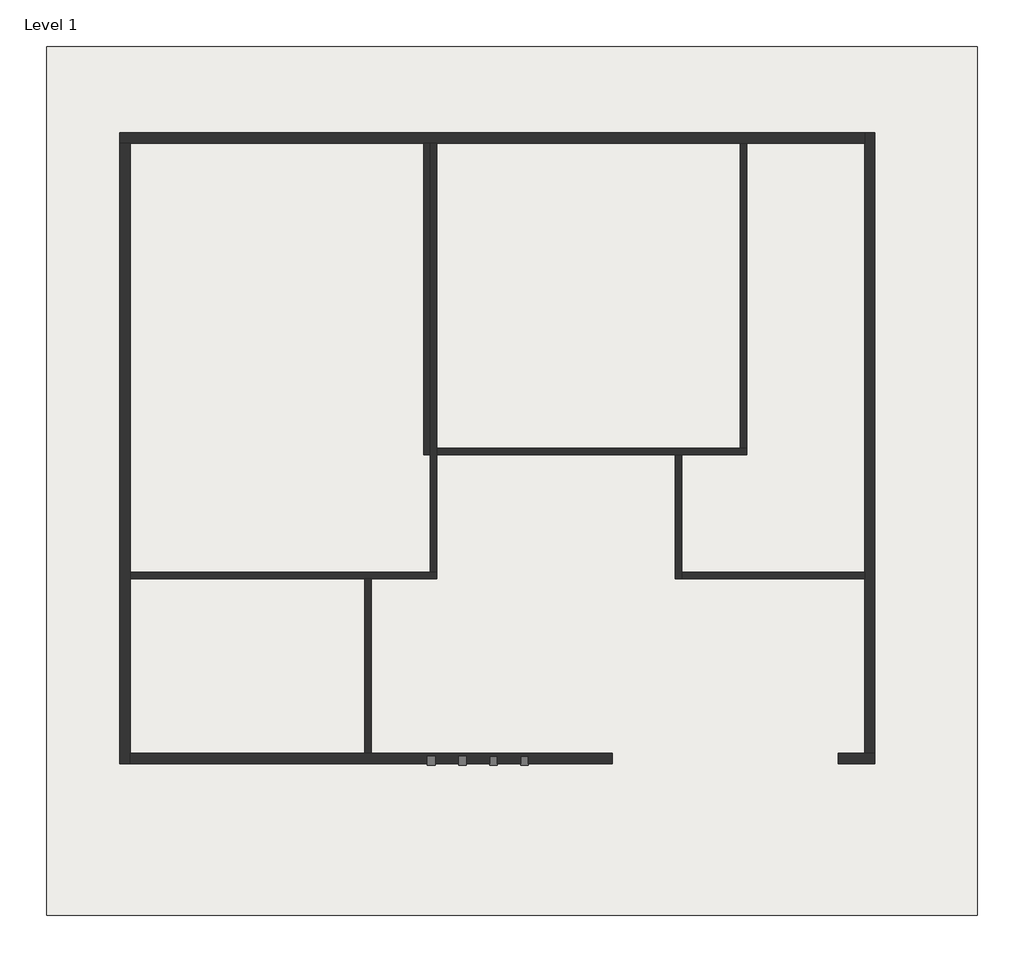
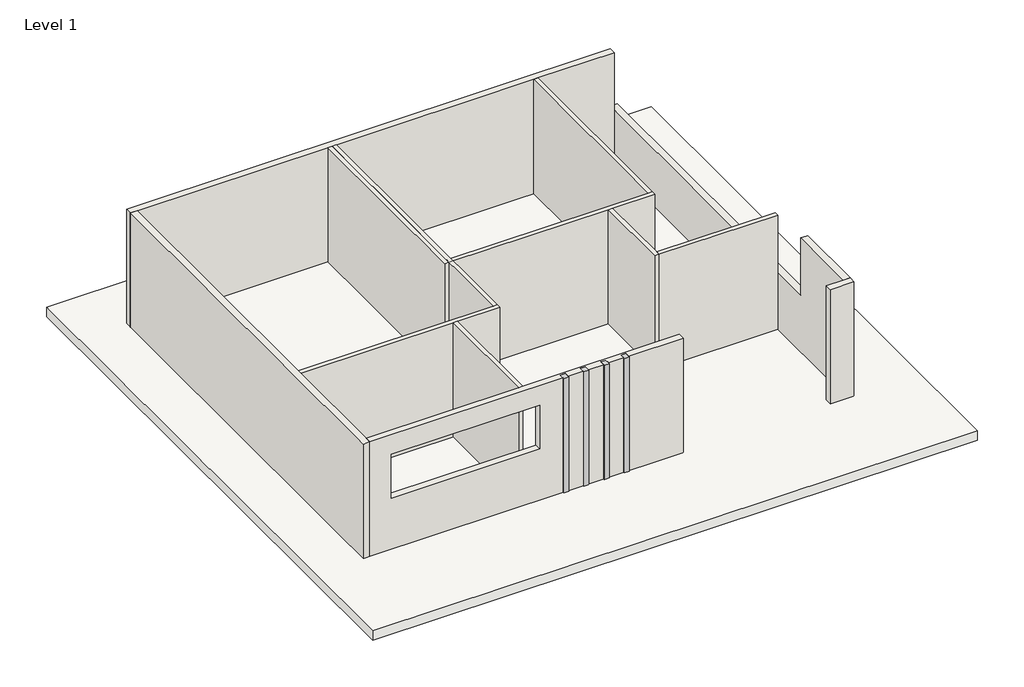
# One storey: 12 walls, 4 proxies, 1 slab.
"""IFC4 building model written with IfcOpenShell, lengths in millimetres."""

from ifc_helpers import new_model, si_unit, frame, origin, origin_with_axes, place, context, project, spatial, polyline, outline, extrude, faceted_brep, element, save

model = new_model("IFC4")

# Units and contexts
model_context = context("Model", 3, world=origin())
ifc_project = project(units=[si_unit("LENGTHUNIT", "METRE", prefix="MILLI")], contexts=[model_context])

# Site, building, storey
site = spatial("IfcSite", under=ifc_project)
building = spatial("IfcBuilding", under=site)
storey = spatial("IfcBuildingStorey", under=building, Name="Level 1", Elevation=0.0)

# Proxies
placement = place(None, origin())
element("IfcBuildingElementProxy", 1, Name="Reveal", ObjectType="Reveal", at=placement, inside=storey, context=model_context, shape_type="SweptSolid", body=[
    extrude(outline(polyline([(-2724.5749149, -2415.4251257), (-2724.5749149, -2232.5451257), (-2572.1749149, -2232.5451257), (-2572.1749149, -2415.4251257), (-2724.5749149, -2415.4251257)])), origin_with_axes(), (0.0, 0.0, 1.0), 3657.6),
])
element("IfcBuildingElementProxy", 2, Name="Reveal", ObjectType="Reveal", at=placement, inside=storey, context=model_context, shape_type="SweptSolid", body=[
    extrude(outline(polyline([(-2114.9749149, -2415.4251257), (-2114.9749149, -2232.5451257), (-1962.5749149, -2232.5451257), (-1962.5749149, -2415.4251257), (-2114.9749149, -2415.4251257)])), origin_with_axes(), (0.0, 0.0, 1.0), 3657.6),
])
element("IfcBuildingElementProxy", 3, Name="Reveal", ObjectType="Reveal", at=placement, inside=storey, context=model_context, shape_type="SweptSolid", body=[
    extrude(outline(polyline([(-1505.3749149, -2415.4251257), (-1505.3749149, -2232.5451257), (-1352.9749149, -2232.5451257), (-1352.9749149, -2415.4251257), (-1505.3749149, -2415.4251257)])), origin_with_axes(), (0.0, 0.0, 1.0), 3657.6),
])
element("IfcBuildingElementProxy", 4, Name="Reveal", ObjectType="Reveal", at=placement, inside=storey, context=model_context, shape_type="SweptSolid", body=[
    extrude(outline(polyline([(-895.7749149, -2415.4251257), (-895.7749149, -2232.5451257), (-743.3749149, -2232.5451257), (-743.3749149, -2415.4251257), (-895.7749149, -2415.4251257)])), origin_with_axes(), (0.0, 0.0, 1.0), 3657.6),
])

# Slab
element("IfcSlab", 5, ObjectType="Generic - 12\"", at=placement, inside=storey, context=model_context, shape_type="SweptSolid", body=[
    extrude(outline(polyline([(8079.4752863, 11705.7296395), (8079.4752863, -5363.0703605), (-10208.5247137, -5363.0703605), (-10208.5247137, 11705.7296395), (8079.4752863, 11705.7296395)])), frame((0.0, 0.0, -304.8), z_axis=(0.0, 0.0, 1.0), x_axis=(1.0, 0.0, 0.0)), (0.0, 0.0, 1.0), 304.8),
])

# Walls
element("IfcWall", 6, ObjectType="Generic - 5\"", at=placement, inside=storey, context=model_context, shape_type="Brep", body=[
    faceted_brep([(-8566.5749149, 1247.2548743, 0.0), (-3956.4749149, 1247.2548743, 0.0), (-3829.4749149, 1247.2548743, 0.0), (-2546.7749149, 1247.2548743, 0.0), (-2546.7749149, 1247.2548743, 3657.6), (-3829.4749149, 1247.2548743, 3657.6), (-3956.4749149, 1247.2548743, 3657.6), (-8566.5749149, 1247.2548743, 3657.6), (-8566.5749149, 1374.2548743, 0.0), (-8566.5749149, 1374.2548743, 3657.6), (-2673.7749149, 1374.2548743, 3657.6), (-2546.7749149, 1374.2548743, 3657.6), (-2546.7749149, 1374.2548743, 0.0), (-2673.7749149, 1374.2548743, 0.0)], [[[0, 1, 2, 3, 4, 5, 6, 7]], [[8, 9, 10, 11, 12, 13]], [[3, 2, 1, 0, 8, 13, 12]], [[7, 6, 5, 4, 11, 10, 9]], [[0, 7, 9, 8]], [[4, 3, 12, 11]]]),
])
element("IfcWall", 7, ObjectType="Generic - 5\"", at=placement, inside=storey, context=model_context, shape_type="SweptSolid", body=[
    extrude(outline(polyline([(-2546.7749149, 9807.0548743), (-2546.7749149, 1374.2548743), (-2673.7749149, 1374.2548743), (-2673.7749149, 9807.0548743), (-2546.7749149, 9807.0548743)])), origin_with_axes(), (0.0, 0.0, 1.0), 3657.6),
])
element("IfcWall", 8, ObjectType="Generic - 5\"", at=placement, inside=storey, context=model_context, shape_type="Brep", body=[
    faceted_brep([(-2800.7749149, 9807.0548743, 0.0), (-2800.7749149, 3685.6548743, 0.0), (-2800.7749149, 3685.6548743, 3657.6), (-2800.7749149, 9807.0548743, 3657.6), (-2673.7749149, 9807.0548743, 0.0), (-2673.7749149, 9807.0548743, 3657.6), (-2673.7749149, 3812.6548743, 3657.6), (-2673.7749149, 3685.6548743, 3657.6), (-2673.7749149, 3685.6548743, 0.0), (-2673.7749149, 3812.6548743, 0.0)], [[[0, 1, 2, 3]], [[4, 5, 6, 7, 8, 9]], [[1, 0, 4, 9, 8]], [[3, 2, 7, 6, 5]], [[0, 3, 5, 4]], [[2, 1, 8, 7]]]),
])
element("IfcWall", 9, ObjectType="Generic - 5\"", at=placement, inside=storey, context=model_context, shape_type="Brep", body=[
    faceted_brep([(-2673.7749149, 3685.6548743, 0.0), (2139.5250851, 3685.6548743, 0.0), (2266.5250851, 3685.6548743, 0.0), (3549.2250851, 3685.6548743, 0.0), (3549.2250851, 3685.6548743, 3657.6), (2266.5250851, 3685.6548743, 3657.6), (2139.5250851, 3685.6548743, 3657.6), (-2673.7749149, 3685.6548743, 3657.6), (-2673.7749149, 3812.6548743, 0.0), (-2673.7749149, 3812.6548743, 3657.6), (3422.2250851, 3812.6548743, 3657.6), (3549.2250851, 3812.6548743, 3657.6), (3549.2250851, 3812.6548743, 0.0), (3422.2250851, 3812.6548743, 0.0)], [[[0, 1, 2, 3, 4, 5, 6, 7]], [[8, 9, 10, 11, 12, 13]], [[3, 2, 1, 0, 8, 13, 12]], [[7, 6, 5, 4, 11, 10, 9]], [[0, 7, 9, 8]], [[4, 3, 12, 11]]]),
])
element("IfcWall", 10, ObjectType="Generic - 5\"", at=placement, inside=storey, context=model_context, shape_type="SweptSolid", body=[
    extrude(outline(polyline([(3549.2250851, 9807.0548743), (3549.2250851, 3812.6548743), (3422.2250851, 3812.6548743), (3422.2250851, 9807.0548743), (3549.2250851, 9807.0548743)])), origin_with_axes(), (0.0, 0.0, 1.0), 3657.6),
])
element("IfcWall", 11, ObjectType="Generic - 5\"", at=placement, inside=storey, context=model_context, shape_type="Brep", body=[
    faceted_brep([(2139.5250851, 3685.6548743, 0.0), (2139.5250851, 1247.2548743, 0.0), (2139.5250851, 1247.2548743, 3657.6), (2139.5250851, 3685.6548743, 3657.6), (2266.5250851, 3685.6548743, 0.0), (2266.5250851, 3685.6548743, 3657.6), (2266.5250851, 1374.2548743, 3657.6), (2266.5250851, 1247.2548743, 3657.6), (2266.5250851, 1247.2548743, 0.0), (2266.5250851, 1374.2548743, 0.0)], [[[0, 1, 2, 3]], [[4, 5, 6, 7, 8, 9]], [[1, 0, 4, 9, 8]], [[3, 2, 7, 6, 5]], [[0, 3, 5, 4]], [[2, 1, 8, 7]]]),
])
element("IfcWall", 12, ObjectType="Generic - 5\"", at=placement, inside=storey, context=model_context, shape_type="SweptSolid", body=[
    extrude(outline(polyline([(5860.6250851, 1247.2548743), (2266.5250851, 1247.2548743), (2266.5250851, 1374.2548743), (5860.6250851, 1374.2548743), (5860.6250851, 1247.2548743)])), origin_with_axes(), (0.0, 0.0, 1.0), 3657.6),
])
element("IfcWall", 13, ObjectType="Generic - 5\"", at=placement, inside=storey, context=model_context, shape_type="SweptSolid", body=[
    extrude(outline(polyline([(-3829.4749149, 1247.2548743), (-3829.4749149, -2181.7451257), (-3956.4749149, -2181.7451257), (-3956.4749149, 1247.2548743), (-3829.4749149, 1247.2548743)])), origin_with_axes(), (0.0, 0.0, 1.0), 3657.6),
])
element("IfcWall", 14, ObjectType="Generic - 8\"", at=placement, inside=storey, context=model_context, shape_type="Brep", body=[
    faceted_brep([(-8769.7749149, 9807.0548743, 0.0), (-8566.5749149, 9807.0548743, 0.0), (-2800.7749149, 9807.0548743, 0.0), (-2673.7749149, 9807.0548743, 0.0), (3422.2250851, 9807.0548743, 0.0), (3549.2250851, 9807.0548743, 0.0), (5860.6250851, 9807.0548743, 0.0), (5860.6250851, 9807.0548743, 3657.6), (3549.2250851, 9807.0548743, 3657.6), (3422.2250851, 9807.0548743, 3657.6), (-2673.7749149, 9807.0548743, 3657.6), (-2800.7749149, 9807.0548743, 3657.6), (-8566.5749149, 9807.0548743, 3657.6), (-8769.7749149, 9807.0548743, 3657.6), (-8769.7749149, 10010.2548743, 0.0), (-8769.7749149, 10010.2548743, 3657.6), (5860.6250851, 10010.2548743, 3657.6), (5860.6250851, 10010.2548743, 1828.8), (5860.6250851, 10010.2548743, 0.0)], [[[0, 1, 2, 3, 4, 5, 6, 7, 8, 9, 10, 11, 12, 13]], [[14, 15, 16, 17, 18]], [[6, 5, 4, 3, 2, 1, 0, 14, 18]], [[0, 13, 15, 14]], [[7, 6, 18, 17, 16]], [[13, 12, 11, 10, 9, 8, 7, 16, 15]]]),
])
element("IfcWall", 15, ObjectType="Generic - 8\"", at=placement, inside=storey, context=model_context, shape_type="Brep", body=[
    faceted_brep([(-8566.5749149, -2384.9451257, 0.0), (-8566.5749149, -2181.7451257, 0.0), (-8566.5749149, 1247.2548743, 0.0), (-8566.5749149, 1374.2548743, 0.0), (-8566.5749149, 9807.0548743, 0.0), (-8566.5749149, 9807.0548743, 3657.6), (-8566.5749149, 1374.2548743, 3657.6), (-8566.5749149, 1247.2548743, 3657.6), (-8566.5749149, -2181.7451257, 3657.6), (-8566.5749149, -2384.9451257, 3657.6), (-8769.7749149, -2384.9451257, 0.0), (-8769.7749149, -2384.9451257, 3657.6), (-8769.7749149, 9807.0548743, 3657.6), (-8769.7749149, 9807.0548743, 0.0)], [[[0, 1, 2, 3, 4, 5, 6, 7, 8, 9]], [[10, 11, 12, 13]], [[4, 3, 2, 1, 0, 10, 13]], [[0, 9, 11, 10]], [[5, 4, 13, 12]], [[9, 8, 7, 6, 5, 12, 11]]]),
])
element("IfcWall", 16, ObjectType="Generic - 8\"", at=placement, inside=storey, context=model_context, shape_type="Brep", body=[
    faceted_brep([(-8566.5749149, -2181.7451257, 0.0), (-8566.5749149, -2181.7451257, 3657.6), (-3956.4749149, -2181.7451257, 3657.6), (-3829.4749149, -2181.7451257, 3657.6), (907.6250851, -2181.7451257, 3657.6), (907.6250851, -2181.7451257, 0.0), (-3829.4749149, -2181.7451257, 0.0), (-3956.4749149, -2181.7451257, 0.0), (-3435.7749149, -2181.7451257, 3037.1162749), (-7920.2332055, -2181.7451257, 3037.1162749), (-7920.2332055, -2181.7451257, 1637.4264186), (-3435.7749149, -2181.7451257, 1637.4264186), (-8566.5749149, -2384.9451257, 3657.6), (-8566.5749149, -2384.9451257, 0.0), (-2724.5749149, -2384.9451257, 0.0), (-2724.5749149, -2384.9451257, 3657.6), (-7920.2332055, -2384.9451257, 3037.1162749), (-3435.7749149, -2384.9451257, 3037.1162749), (-3435.7749149, -2384.9451257, 1637.4264186), (-7920.2332055, -2384.9451257, 1637.4264186), (-2572.1749149, -2384.9451257, 3657.6), (-2572.1749149, -2384.9451257, 0.0), (-2114.9749149, -2384.9451257, 0.0), (-2114.9749149, -2384.9451257, 3657.6), (-1962.5749149, -2384.9451257, 3657.6), (-1962.5749149, -2384.9451257, 0.0), (-1505.3749149, -2384.9451257, 0.0), (-1505.3749149, -2384.9451257, 3657.6), (-1352.9749149, -2384.9451257, 3657.6), (-1352.9749149, -2384.9451257, 0.0), (-895.7749149, -2384.9451257, 0.0), (-895.7749149, -2384.9451257, 3657.6), (907.6250851, -2384.9451257, 0.0), (907.6250851, -2384.9451257, 3657.6), (-743.3749149, -2384.9451257, 3657.6), (-743.3749149, -2384.9451257, 0.0), (-2724.5749149, -2232.5451257, 0.0), (-2724.5749149, -2232.5451257, 3657.6), (-2572.1749149, -2232.5451257, 0.0), (-2572.1749149, -2232.5451257, 3657.6), (-2114.9749149, -2232.5451257, 0.0), (-2114.9749149, -2232.5451257, 3657.6), (-1962.5749149, -2232.5451257, 0.0), (-1962.5749149, -2232.5451257, 3657.6), (-1505.3749149, -2232.5451257, 0.0), (-1505.3749149, -2232.5451257, 3657.6), (-1352.9749149, -2232.5451257, 0.0), (-1352.9749149, -2232.5451257, 3657.6), (-895.7749149, -2232.5451257, 0.0), (-895.7749149, -2232.5451257, 3657.6), (-743.3749149, -2232.5451257, 0.0), (-743.3749149, -2232.5451257, 3657.6)], [[[0, 1, 2, 3, 4, 5, 6, 7], [8, 9, 10, 11]], [[12, 13, 14, 15], [16, 17, 18, 19]], [[20, 21, 22, 23]], [[24, 25, 26, 27]], [[28, 29, 30, 31]], [[32, 33, 34, 35]], [[1, 0, 13, 12]], [[9, 8, 17, 16]], [[10, 9, 16, 19]], [[11, 10, 19, 18]], [[8, 11, 18, 17]], [[36, 37, 15, 14]], [[37, 36, 38, 39]], [[39, 38, 21, 20]], [[40, 41, 23, 22]], [[41, 40, 42, 43]], [[43, 42, 25, 24]], [[44, 45, 27, 26]], [[45, 44, 46, 47]], [[47, 46, 29, 28]], [[48, 49, 31, 30]], [[49, 48, 50, 51]], [[51, 50, 35, 34]], [[5, 4, 33, 32]], [[0, 7, 6, 5, 32, 35, 50, 48, 30, 29, 46, 44, 26, 25, 42, 40, 22, 21, 38, 36, 14, 13]], [[4, 3, 2, 1, 12, 15, 37, 39, 20, 23, 41, 43, 24, 27, 45, 47, 28, 31, 49, 51, 34, 33]]]),
    faceted_brep([(6063.8250851, -2181.7451257, 3657.6), (6063.8250851, -2181.7451257, 0.0), (5860.6250851, -2181.7451257, 0.0), (5347.1745768, -2181.7451257, 0.0), (5347.1745768, -2181.7451257, 3657.6), (5860.6250851, -2181.7451257, 3657.6), (6063.8250851, -2384.9451257, 0.0), (6063.8250851, -2384.9451257, 3657.6), (5347.1745768, -2384.9451257, 3657.6), (5347.1745768, -2384.9451257, 0.0)], [[[0, 1, 2, 3, 4, 5]], [[6, 7, 8, 9]], [[1, 0, 7, 6]], [[3, 2, 1, 6, 9]], [[4, 3, 9, 8]], [[0, 5, 4, 8, 7]]]),
])
element("IfcWall", 17, ObjectType="Generic - 8\"", at=placement, inside=storey, context=model_context, shape_type="Brep", body=[
    faceted_brep([(5860.6250851, 10010.2548743, 0.0), (5860.6250851, 9807.0548743, 0.0), (5860.6250851, 1374.2548743, 0.0), (5860.6250851, 1247.2548743, 0.0), (5860.6250851, 40.7548743, 0.0), (5860.6250851, -2181.7451257, 0.0), (5860.6250851, -2181.7451257, 3657.6), (5860.6250851, 40.7548743, 3657.6), (5860.6250851, 40.7548743, 1828.8), (5860.6250851, 10010.2548743, 1828.8), (6063.8250851, 10010.2548743, 0.0), (6063.8250851, 10010.2548743, 1828.8), (6063.8250851, 40.7548743, 1828.8), (6063.8250851, 40.7548743, 3657.6), (6063.8250851, -2181.7451257, 3657.6), (6063.8250851, -2181.7451257, 0.0), (6063.8250851, 40.7548743, 0.0)], [[[0, 1, 2, 3, 4, 5, 6, 7, 8, 9]], [[10, 11, 12, 13, 14, 15, 16]], [[0, 9, 11, 10]], [[6, 5, 15, 14]], [[4, 3, 2, 1, 0, 10, 16]], [[8, 7, 13, 12]], [[5, 4, 16, 15]], [[9, 8, 12, 11]], [[7, 6, 14, 13]]]),
])

save(model, "model.ifc")

# Revit data of these elements
# Type "Generic - 12\""
#   Assembly Code = "B1010"
#   Function = 0
#   Layers, outside or top first: 1' - 0" no material (function 1)
# Type "Generic - 5\""
#   Assembly Code = "B2010"
#   Layers, outside or top first: 0' - 5" no material (function 1)
# Type "Generic - 8\""
#   Assembly Code = "B2010"
#   Layers, outside or top first: 0' - 8" no material (function 1)
# Element 5 (IfcSlab, "Generic - 12\"")
#   Height Offset From Level = 0' - 0"
#   Phase Created = New Construction
#   Materials on its faces: "Default Floor"
# Elements 6, 7, 8, 9, 10, 11, 12, 13 (IfcWall, "Generic - 5\"")
#   Top Offset = 0' - 0"
#   Base Offset = 0' - 0"
#   wall height = 12' - 0"
#   Phase Created = New Construction
#   Base Constraint = Level 1
#   Top Constraint = Level 2
#   Materials on its faces: "Default Wall"
# Elements 14, 15, 16, 17 (IfcWall, "Generic - 8\"")
#   Top Offset = 0' - 0"
#   Base Offset = 0' - 0"
#   Unconnected Height = 12' - 0"
#   wall height = 12' - 0"
#   Phase Created = New Construction
#   Base Constraint = Level 1
#   Materials on its faces: "Default Wall"
# Materials
#   "Default Floor": colour RGB 128 128 128, transparency 0
#   "Default Wall": colour RGB 128 128 128, transparency 0
